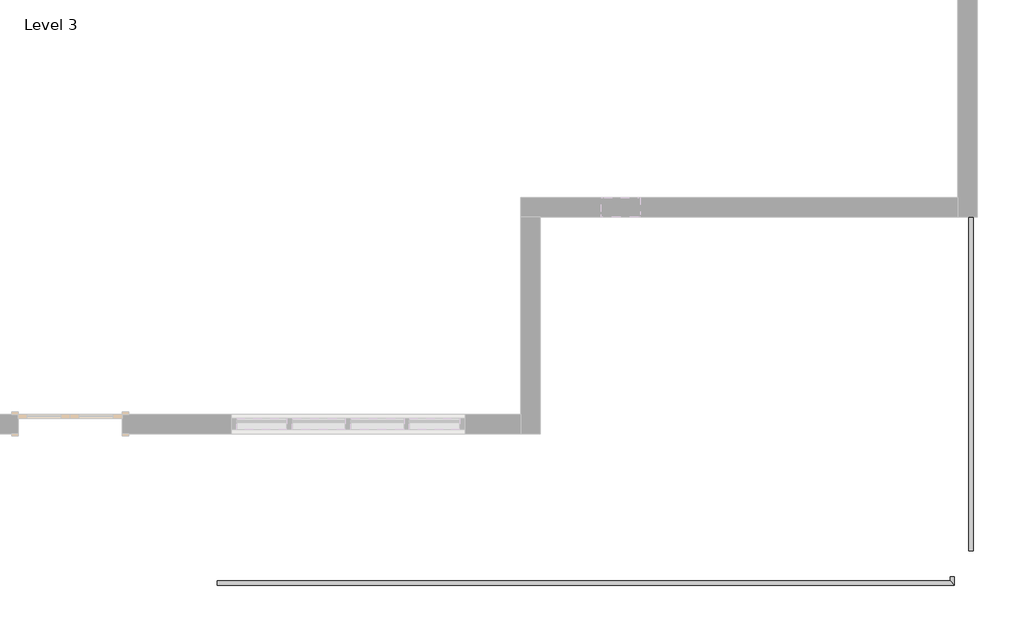
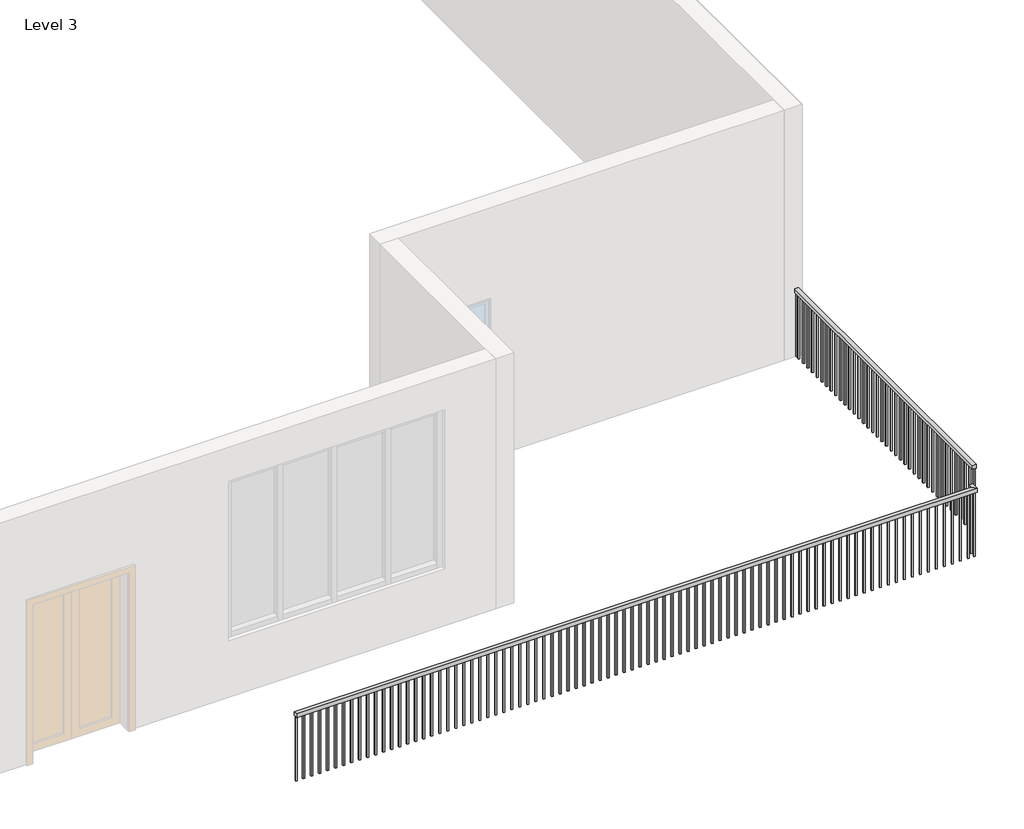
# One storey, part 2 of 2: 2 railings.
"""IFC4 building model written with IfcOpenShell, lengths in millimetres."""

from ifc_helpers import new_model, si_unit, frame, origin, place, context, project, spatial, polyline, outline, extrude, faceted_brep, element, save

model = new_model("IFC4")

# Units and contexts
model_context = context("Model", 3, world=origin())
ifc_project = project(units=[si_unit("LENGTHUNIT", "METRE", prefix="MILLI")], contexts=[model_context])

# Site, building, storey
site = spatial("IfcSite", under=ifc_project)
building = spatial("IfcBuilding", under=site)
storey = spatial("IfcBuildingStorey", under=building, Name="Level 3", Elevation=4114.8)

# Railings
placement = place(None, origin())
element("IfcRailing", 1, ObjectType="Handrail - Rectangular", at=placement, inside=storey, context=model_context, shape_type="SolidModel", body=[
    faceted_brep([(-103.6484006, -4656.0372669, 5029.2), (-103.6484006, -4656.0372669, 4978.4), (-103.6484006, -4706.8372669, 4978.4), (-103.6484006, -4706.8372669, 5029.2), (8481.5515994, -4656.0372669, 5029.2), (8481.5515994, -4656.0372669, 4978.4), (8532.3515994, -4706.8372669, 4978.4), (8532.3515994, -4706.8372669, 5029.2), (8481.5515994, -4605.2372669, 5029.2), (8532.3515994, -4605.2372669, 5029.2), (8532.3515994, -4605.2372669, 4978.4), (8481.5515994, -4605.2372669, 4978.4)], [[[0, 1, 2, 3]], [[1, 0, 4, 5]], [[2, 1, 5, 6]], [[3, 2, 6, 7]], [[0, 3, 7, 4]], [[8, 9, 10, 11]], [[5, 4, 8, 11]], [[6, 5, 11, 10]], [[7, 6, 10, 9]], [[4, 7, 9, 8]]]),
    extrude(outline(polyline([(8421.2265994, -4690.9622669), (8421.2265994, -4671.9122669), (8440.2765994, -4671.9122669), (8440.2765994, -4690.9622669), (8421.2265994, -4690.9622669)])), frame((0.0, 0.0, 4114.8), z_axis=(0.0, 0.0, 1.0), x_axis=(1.0, 0.0, 0.0)), (0.0, 0.0, 1.0), 863.6),
    extrude(outline(polyline([(8319.6265994, -4690.9622669), (8319.6265994, -4671.9122669), (8338.6765994, -4671.9122669), (8338.6765994, -4690.9622669), (8319.6265994, -4690.9622669)])), frame((0.0, 0.0, 4114.8), z_axis=(0.0, 0.0, 1.0), x_axis=(1.0, 0.0, 0.0)), (0.0, 0.0, 1.0), 863.6),
    extrude(outline(polyline([(8218.0265994, -4690.9622669), (8218.0265994, -4671.9122669), (8237.0765994, -4671.9122669), (8237.0765994, -4690.9622669), (8218.0265994, -4690.9622669)])), frame((0.0, 0.0, 4114.8), z_axis=(0.0, 0.0, 1.0), x_axis=(1.0, 0.0, 0.0)), (0.0, 0.0, 1.0), 863.6),
    extrude(outline(polyline([(8116.4265994, -4690.9622669), (8116.4265994, -4671.9122669), (8135.4765994, -4671.9122669), (8135.4765994, -4690.9622669), (8116.4265994, -4690.9622669)])), frame((0.0, 0.0, 4114.8), z_axis=(0.0, 0.0, 1.0), x_axis=(1.0, 0.0, 0.0)), (0.0, 0.0, 1.0), 863.6),
    extrude(outline(polyline([(8014.8265994, -4690.9622669), (8014.8265994, -4671.9122669), (8033.8765994, -4671.9122669), (8033.8765994, -4690.9622669), (8014.8265994, -4690.9622669)])), frame((0.0, 0.0, 4114.8), z_axis=(0.0, 0.0, 1.0), x_axis=(1.0, 0.0, 0.0)), (0.0, 0.0, 1.0), 863.6),
    extrude(outline(polyline([(7913.2265994, -4690.9622669), (7913.2265994, -4671.9122669), (7932.2765994, -4671.9122669), (7932.2765994, -4690.9622669), (7913.2265994, -4690.9622669)])), frame((0.0, 0.0, 4114.8), z_axis=(0.0, 0.0, 1.0), x_axis=(1.0, 0.0, 0.0)), (0.0, 0.0, 1.0), 863.6),
    extrude(outline(polyline([(7811.6265994, -4690.9622669), (7811.6265994, -4671.9122669), (7830.6765994, -4671.9122669), (7830.6765994, -4690.9622669), (7811.6265994, -4690.9622669)])), frame((0.0, 0.0, 4114.8), z_axis=(0.0, 0.0, 1.0), x_axis=(1.0, 0.0, 0.0)), (0.0, 0.0, 1.0), 863.6),
    extrude(outline(polyline([(7710.0265994, -4690.9622669), (7710.0265994, -4671.9122669), (7729.0765994, -4671.9122669), (7729.0765994, -4690.9622669), (7710.0265994, -4690.9622669)])), frame((0.0, 0.0, 4114.8), z_axis=(0.0, 0.0, 1.0), x_axis=(1.0, 0.0, 0.0)), (0.0, 0.0, 1.0), 863.6),
    extrude(outline(polyline([(7608.4265994, -4690.9622669), (7608.4265994, -4671.9122669), (7627.4765994, -4671.9122669), (7627.4765994, -4690.9622669), (7608.4265994, -4690.9622669)])), frame((0.0, 0.0, 4114.8), z_axis=(0.0, 0.0, 1.0), x_axis=(1.0, 0.0, 0.0)), (0.0, 0.0, 1.0), 863.6),
    extrude(outline(polyline([(7506.8265994, -4690.9622669), (7506.8265994, -4671.9122669), (7525.8765994, -4671.9122669), (7525.8765994, -4690.9622669), (7506.8265994, -4690.9622669)])), frame((0.0, 0.0, 4114.8), z_axis=(0.0, 0.0, 1.0), x_axis=(1.0, 0.0, 0.0)), (0.0, 0.0, 1.0), 863.6),
    extrude(outline(polyline([(7405.2265994, -4690.9622669), (7405.2265994, -4671.9122669), (7424.2765994, -4671.9122669), (7424.2765994, -4690.9622669), (7405.2265994, -4690.9622669)])), frame((0.0, 0.0, 4114.8), z_axis=(0.0, 0.0, 1.0), x_axis=(1.0, 0.0, 0.0)), (0.0, 0.0, 1.0), 863.6),
    extrude(outline(polyline([(7303.6265994, -4690.9622669), (7303.6265994, -4671.9122669), (7322.6765994, -4671.9122669), (7322.6765994, -4690.9622669), (7303.6265994, -4690.9622669)])), frame((0.0, 0.0, 4114.8), z_axis=(0.0, 0.0, 1.0), x_axis=(1.0, 0.0, 0.0)), (0.0, 0.0, 1.0), 863.6),
    extrude(outline(polyline([(7202.0265994, -4690.9622669), (7202.0265994, -4671.9122669), (7221.0765994, -4671.9122669), (7221.0765994, -4690.9622669), (7202.0265994, -4690.9622669)])), frame((0.0, 0.0, 4114.8), z_axis=(0.0, 0.0, 1.0), x_axis=(1.0, 0.0, 0.0)), (0.0, 0.0, 1.0), 863.6),
    extrude(outline(polyline([(7100.4265994, -4690.9622669), (7100.4265994, -4671.9122669), (7119.4765994, -4671.9122669), (7119.4765994, -4690.9622669), (7100.4265994, -4690.9622669)])), frame((0.0, 0.0, 4114.8), z_axis=(0.0, 0.0, 1.0), x_axis=(1.0, 0.0, 0.0)), (0.0, 0.0, 1.0), 863.6),
    extrude(outline(polyline([(6998.8265994, -4690.9622669), (6998.8265994, -4671.9122669), (7017.8765994, -4671.9122669), (7017.8765994, -4690.9622669), (6998.8265994, -4690.9622669)])), frame((0.0, 0.0, 4114.8), z_axis=(0.0, 0.0, 1.0), x_axis=(1.0, 0.0, 0.0)), (0.0, 0.0, 1.0), 863.6),
    extrude(outline(polyline([(6897.2265994, -4690.9622669), (6897.2265994, -4671.9122669), (6916.2765994, -4671.9122669), (6916.2765994, -4690.9622669), (6897.2265994, -4690.9622669)])), frame((0.0, 0.0, 4114.8), z_axis=(0.0, 0.0, 1.0), x_axis=(1.0, 0.0, 0.0)), (0.0, 0.0, 1.0), 863.6),
    extrude(outline(polyline([(6795.6265994, -4690.9622669), (6795.6265994, -4671.9122669), (6814.6765994, -4671.9122669), (6814.6765994, -4690.9622669), (6795.6265994, -4690.9622669)])), frame((0.0, 0.0, 4114.8), z_axis=(0.0, 0.0, 1.0), x_axis=(1.0, 0.0, 0.0)), (0.0, 0.0, 1.0), 863.6),
    extrude(outline(polyline([(6694.0265994, -4690.9622669), (6694.0265994, -4671.9122669), (6713.0765994, -4671.9122669), (6713.0765994, -4690.9622669), (6694.0265994, -4690.9622669)])), frame((0.0, 0.0, 4114.8), z_axis=(0.0, 0.0, 1.0), x_axis=(1.0, 0.0, 0.0)), (0.0, 0.0, 1.0), 863.6),
    extrude(outline(polyline([(6592.4265994, -4690.9622669), (6592.4265994, -4671.9122669), (6611.4765994, -4671.9122669), (6611.4765994, -4690.9622669), (6592.4265994, -4690.9622669)])), frame((0.0, 0.0, 4114.8), z_axis=(0.0, 0.0, 1.0), x_axis=(1.0, 0.0, 0.0)), (0.0, 0.0, 1.0), 863.6),
    extrude(outline(polyline([(6490.8265994, -4690.9622669), (6490.8265994, -4671.9122669), (6509.8765994, -4671.9122669), (6509.8765994, -4690.9622669), (6490.8265994, -4690.9622669)])), frame((0.0, 0.0, 4114.8), z_axis=(0.0, 0.0, 1.0), x_axis=(1.0, 0.0, 0.0)), (0.0, 0.0, 1.0), 863.6),
    extrude(outline(polyline([(6389.2265994, -4690.9622669), (6389.2265994, -4671.9122669), (6408.2765994, -4671.9122669), (6408.2765994, -4690.9622669), (6389.2265994, -4690.9622669)])), frame((0.0, 0.0, 4114.8), z_axis=(0.0, 0.0, 1.0), x_axis=(1.0, 0.0, 0.0)), (0.0, 0.0, 1.0), 863.6),
    extrude(outline(polyline([(6287.6265994, -4690.9622669), (6287.6265994, -4671.9122669), (6306.6765994, -4671.9122669), (6306.6765994, -4690.9622669), (6287.6265994, -4690.9622669)])), frame((0.0, 0.0, 4114.8), z_axis=(0.0, 0.0, 1.0), x_axis=(1.0, 0.0, 0.0)), (0.0, 0.0, 1.0), 863.6),
    extrude(outline(polyline([(6186.0265994, -4690.9622669), (6186.0265994, -4671.9122669), (6205.0765994, -4671.9122669), (6205.0765994, -4690.9622669), (6186.0265994, -4690.9622669)])), frame((0.0, 0.0, 4114.8), z_axis=(0.0, 0.0, 1.0), x_axis=(1.0, 0.0, 0.0)), (0.0, 0.0, 1.0), 863.6),
    extrude(outline(polyline([(6084.4265994, -4690.9622669), (6084.4265994, -4671.9122669), (6103.4765994, -4671.9122669), (6103.4765994, -4690.9622669), (6084.4265994, -4690.9622669)])), frame((0.0, 0.0, 4114.8), z_axis=(0.0, 0.0, 1.0), x_axis=(1.0, 0.0, 0.0)), (0.0, 0.0, 1.0), 863.6),
    extrude(outline(polyline([(5982.8265994, -4690.9622669), (5982.8265994, -4671.9122669), (6001.8765994, -4671.9122669), (6001.8765994, -4690.9622669), (5982.8265994, -4690.9622669)])), frame((0.0, 0.0, 4114.8), z_axis=(0.0, 0.0, 1.0), x_axis=(1.0, 0.0, 0.0)), (0.0, 0.0, 1.0), 863.6),
    extrude(outline(polyline([(5881.2265994, -4690.9622669), (5881.2265994, -4671.9122669), (5900.2765994, -4671.9122669), (5900.2765994, -4690.9622669), (5881.2265994, -4690.9622669)])), frame((0.0, 0.0, 4114.8), z_axis=(0.0, 0.0, 1.0), x_axis=(1.0, 0.0, 0.0)), (0.0, 0.0, 1.0), 863.6),
    extrude(outline(polyline([(5779.6265994, -4690.9622669), (5779.6265994, -4671.9122669), (5798.6765994, -4671.9122669), (5798.6765994, -4690.9622669), (5779.6265994, -4690.9622669)])), frame((0.0, 0.0, 4114.8), z_axis=(0.0, 0.0, 1.0), x_axis=(1.0, 0.0, 0.0)), (0.0, 0.0, 1.0), 863.6),
    extrude(outline(polyline([(5678.0265994, -4690.9622669), (5678.0265994, -4671.9122669), (5697.0765994, -4671.9122669), (5697.0765994, -4690.9622669), (5678.0265994, -4690.9622669)])), frame((0.0, 0.0, 4114.8), z_axis=(0.0, 0.0, 1.0), x_axis=(1.0, 0.0, 0.0)), (0.0, 0.0, 1.0), 863.6),
    extrude(outline(polyline([(5576.4265994, -4690.9622669), (5576.4265994, -4671.9122669), (5595.4765994, -4671.9122669), (5595.4765994, -4690.9622669), (5576.4265994, -4690.9622669)])), frame((0.0, 0.0, 4114.8), z_axis=(0.0, 0.0, 1.0), x_axis=(1.0, 0.0, 0.0)), (0.0, 0.0, 1.0), 863.6),
    extrude(outline(polyline([(5474.8265994, -4690.9622669), (5474.8265994, -4671.9122669), (5493.8765994, -4671.9122669), (5493.8765994, -4690.9622669), (5474.8265994, -4690.9622669)])), frame((0.0, 0.0, 4114.8), z_axis=(0.0, 0.0, 1.0), x_axis=(1.0, 0.0, 0.0)), (0.0, 0.0, 1.0), 863.6),
    extrude(outline(polyline([(5373.2265994, -4690.9622669), (5373.2265994, -4671.9122669), (5392.2765994, -4671.9122669), (5392.2765994, -4690.9622669), (5373.2265994, -4690.9622669)])), frame((0.0, 0.0, 4114.8), z_axis=(0.0, 0.0, 1.0), x_axis=(1.0, 0.0, 0.0)), (0.0, 0.0, 1.0), 863.6),
    extrude(outline(polyline([(5271.6265994, -4690.9622669), (5271.6265994, -4671.9122669), (5290.6765994, -4671.9122669), (5290.6765994, -4690.9622669), (5271.6265994, -4690.9622669)])), frame((0.0, 0.0, 4114.8), z_axis=(0.0, 0.0, 1.0), x_axis=(1.0, 0.0, 0.0)), (0.0, 0.0, 1.0), 863.6),
    extrude(outline(polyline([(5170.0265994, -4690.9622669), (5170.0265994, -4671.9122669), (5189.0765994, -4671.9122669), (5189.0765994, -4690.9622669), (5170.0265994, -4690.9622669)])), frame((0.0, 0.0, 4114.8), z_axis=(0.0, 0.0, 1.0), x_axis=(1.0, 0.0, 0.0)), (0.0, 0.0, 1.0), 863.6),
    extrude(outline(polyline([(5068.4265994, -4690.9622669), (5068.4265994, -4671.9122669), (5087.4765994, -4671.9122669), (5087.4765994, -4690.9622669), (5068.4265994, -4690.9622669)])), frame((0.0, 0.0, 4114.8), z_axis=(0.0, 0.0, 1.0), x_axis=(1.0, 0.0, 0.0)), (0.0, 0.0, 1.0), 863.6),
    extrude(outline(polyline([(4966.8265994, -4690.9622669), (4966.8265994, -4671.9122669), (4985.8765994, -4671.9122669), (4985.8765994, -4690.9622669), (4966.8265994, -4690.9622669)])), frame((0.0, 0.0, 4114.8), z_axis=(0.0, 0.0, 1.0), x_axis=(1.0, 0.0, 0.0)), (0.0, 0.0, 1.0), 863.6),
    extrude(outline(polyline([(4865.2265994, -4690.9622669), (4865.2265994, -4671.9122669), (4884.2765994, -4671.9122669), (4884.2765994, -4690.9622669), (4865.2265994, -4690.9622669)])), frame((0.0, 0.0, 4114.8), z_axis=(0.0, 0.0, 1.0), x_axis=(1.0, 0.0, 0.0)), (0.0, 0.0, 1.0), 863.6),
    extrude(outline(polyline([(4763.6265994, -4690.9622669), (4763.6265994, -4671.9122669), (4782.6765994, -4671.9122669), (4782.6765994, -4690.9622669), (4763.6265994, -4690.9622669)])), frame((0.0, 0.0, 4114.8), z_axis=(0.0, 0.0, 1.0), x_axis=(1.0, 0.0, 0.0)), (0.0, 0.0, 1.0), 863.6),
    extrude(outline(polyline([(4662.0265994, -4690.9622669), (4662.0265994, -4671.9122669), (4681.0765994, -4671.9122669), (4681.0765994, -4690.9622669), (4662.0265994, -4690.9622669)])), frame((0.0, 0.0, 4114.8), z_axis=(0.0, 0.0, 1.0), x_axis=(1.0, 0.0, 0.0)), (0.0, 0.0, 1.0), 863.6),
    extrude(outline(polyline([(4560.4265994, -4690.9622669), (4560.4265994, -4671.9122669), (4579.4765994, -4671.9122669), (4579.4765994, -4690.9622669), (4560.4265994, -4690.9622669)])), frame((0.0, 0.0, 4114.8), z_axis=(0.0, 0.0, 1.0), x_axis=(1.0, 0.0, 0.0)), (0.0, 0.0, 1.0), 863.6),
    extrude(outline(polyline([(4458.8265994, -4690.9622669), (4458.8265994, -4671.9122669), (4477.8765994, -4671.9122669), (4477.8765994, -4690.9622669), (4458.8265994, -4690.9622669)])), frame((0.0, 0.0, 4114.8), z_axis=(0.0, 0.0, 1.0), x_axis=(1.0, 0.0, 0.0)), (0.0, 0.0, 1.0), 863.6),
    extrude(outline(polyline([(4357.2265994, -4690.9622669), (4357.2265994, -4671.9122669), (4376.2765994, -4671.9122669), (4376.2765994, -4690.9622669), (4357.2265994, -4690.9622669)])), frame((0.0, 0.0, 4114.8), z_axis=(0.0, 0.0, 1.0), x_axis=(1.0, 0.0, 0.0)), (0.0, 0.0, 1.0), 863.6),
    extrude(outline(polyline([(4255.6265994, -4690.9622669), (4255.6265994, -4671.9122669), (4274.6765994, -4671.9122669), (4274.6765994, -4690.9622669), (4255.6265994, -4690.9622669)])), frame((0.0, 0.0, 4114.8), z_axis=(0.0, 0.0, 1.0), x_axis=(1.0, 0.0, 0.0)), (0.0, 0.0, 1.0), 863.6),
    extrude(outline(polyline([(4154.0265994, -4690.9622669), (4154.0265994, -4671.9122669), (4173.0765994, -4671.9122669), (4173.0765994, -4690.9622669), (4154.0265994, -4690.9622669)])), frame((0.0, 0.0, 4114.8), z_axis=(0.0, 0.0, 1.0), x_axis=(1.0, 0.0, 0.0)), (0.0, 0.0, 1.0), 863.6),
    extrude(outline(polyline([(4052.4265994, -4690.9622669), (4052.4265994, -4671.9122669), (4071.4765994, -4671.9122669), (4071.4765994, -4690.9622669), (4052.4265994, -4690.9622669)])), frame((0.0, 0.0, 4114.8), z_axis=(0.0, 0.0, 1.0), x_axis=(1.0, 0.0, 0.0)), (0.0, 0.0, 1.0), 863.6),
    extrude(outline(polyline([(3950.8265994, -4690.9622669), (3950.8265994, -4671.9122669), (3969.8765994, -4671.9122669), (3969.8765994, -4690.9622669), (3950.8265994, -4690.9622669)])), frame((0.0, 0.0, 4114.8), z_axis=(0.0, 0.0, 1.0), x_axis=(1.0, 0.0, 0.0)), (0.0, 0.0, 1.0), 863.6),
    extrude(outline(polyline([(3849.2265994, -4690.9622669), (3849.2265994, -4671.9122669), (3868.2765994, -4671.9122669), (3868.2765994, -4690.9622669), (3849.2265994, -4690.9622669)])), frame((0.0, 0.0, 4114.8), z_axis=(0.0, 0.0, 1.0), x_axis=(1.0, 0.0, 0.0)), (0.0, 0.0, 1.0), 863.6),
    extrude(outline(polyline([(3747.6265994, -4690.9622669), (3747.6265994, -4671.9122669), (3766.6765994, -4671.9122669), (3766.6765994, -4690.9622669), (3747.6265994, -4690.9622669)])), frame((0.0, 0.0, 4114.8), z_axis=(0.0, 0.0, 1.0), x_axis=(1.0, 0.0, 0.0)), (0.0, 0.0, 1.0), 863.6),
    extrude(outline(polyline([(3646.0265994, -4690.9622669), (3646.0265994, -4671.9122669), (3665.0765994, -4671.9122669), (3665.0765994, -4690.9622669), (3646.0265994, -4690.9622669)])), frame((0.0, 0.0, 4114.8), z_axis=(0.0, 0.0, 1.0), x_axis=(1.0, 0.0, 0.0)), (0.0, 0.0, 1.0), 863.6),
    extrude(outline(polyline([(3544.4265994, -4690.9622669), (3544.4265994, -4671.9122669), (3563.4765994, -4671.9122669), (3563.4765994, -4690.9622669), (3544.4265994, -4690.9622669)])), frame((0.0, 0.0, 4114.8), z_axis=(0.0, 0.0, 1.0), x_axis=(1.0, 0.0, 0.0)), (0.0, 0.0, 1.0), 863.6),
    extrude(outline(polyline([(3442.8265994, -4690.9622669), (3442.8265994, -4671.9122669), (3461.8765994, -4671.9122669), (3461.8765994, -4690.9622669), (3442.8265994, -4690.9622669)])), frame((0.0, 0.0, 4114.8), z_axis=(0.0, 0.0, 1.0), x_axis=(1.0, 0.0, 0.0)), (0.0, 0.0, 1.0), 863.6),
    extrude(outline(polyline([(3341.2265994, -4690.9622669), (3341.2265994, -4671.9122669), (3360.2765994, -4671.9122669), (3360.2765994, -4690.9622669), (3341.2265994, -4690.9622669)])), frame((0.0, 0.0, 4114.8), z_axis=(0.0, 0.0, 1.0), x_axis=(1.0, 0.0, 0.0)), (0.0, 0.0, 1.0), 863.6),
    extrude(outline(polyline([(3239.6265994, -4690.9622669), (3239.6265994, -4671.9122669), (3258.6765994, -4671.9122669), (3258.6765994, -4690.9622669), (3239.6265994, -4690.9622669)])), frame((0.0, 0.0, 4114.8), z_axis=(0.0, 0.0, 1.0), x_axis=(1.0, 0.0, 0.0)), (0.0, 0.0, 1.0), 863.6),
    extrude(outline(polyline([(3138.0265994, -4690.9622669), (3138.0265994, -4671.9122669), (3157.0765994, -4671.9122669), (3157.0765994, -4690.9622669), (3138.0265994, -4690.9622669)])), frame((0.0, 0.0, 4114.8), z_axis=(0.0, 0.0, 1.0), x_axis=(1.0, 0.0, 0.0)), (0.0, 0.0, 1.0), 863.6),
    extrude(outline(polyline([(3036.4265994, -4690.9622669), (3036.4265994, -4671.9122669), (3055.4765994, -4671.9122669), (3055.4765994, -4690.9622669), (3036.4265994, -4690.9622669)])), frame((0.0, 0.0, 4114.8), z_axis=(0.0, 0.0, 1.0), x_axis=(1.0, 0.0, 0.0)), (0.0, 0.0, 1.0), 863.6),
    extrude(outline(polyline([(2934.8265994, -4690.9622669), (2934.8265994, -4671.9122669), (2953.8765994, -4671.9122669), (2953.8765994, -4690.9622669), (2934.8265994, -4690.9622669)])), frame((0.0, 0.0, 4114.8), z_axis=(0.0, 0.0, 1.0), x_axis=(1.0, 0.0, 0.0)), (0.0, 0.0, 1.0), 863.6),
    extrude(outline(polyline([(2833.2265994, -4690.9622669), (2833.2265994, -4671.9122669), (2852.2765994, -4671.9122669), (2852.2765994, -4690.9622669), (2833.2265994, -4690.9622669)])), frame((0.0, 0.0, 4114.8), z_axis=(0.0, 0.0, 1.0), x_axis=(1.0, 0.0, 0.0)), (0.0, 0.0, 1.0), 863.6),
    extrude(outline(polyline([(2731.6265994, -4690.9622669), (2731.6265994, -4671.9122669), (2750.6765994, -4671.9122669), (2750.6765994, -4690.9622669), (2731.6265994, -4690.9622669)])), frame((0.0, 0.0, 4114.8), z_axis=(0.0, 0.0, 1.0), x_axis=(1.0, 0.0, 0.0)), (0.0, 0.0, 1.0), 863.6),
    extrude(outline(polyline([(2630.0265994, -4690.9622669), (2630.0265994, -4671.9122669), (2649.0765994, -4671.9122669), (2649.0765994, -4690.9622669), (2630.0265994, -4690.9622669)])), frame((0.0, 0.0, 4114.8), z_axis=(0.0, 0.0, 1.0), x_axis=(1.0, 0.0, 0.0)), (0.0, 0.0, 1.0), 863.6),
    extrude(outline(polyline([(2528.4265994, -4690.9622669), (2528.4265994, -4671.9122669), (2547.4765994, -4671.9122669), (2547.4765994, -4690.9622669), (2528.4265994, -4690.9622669)])), frame((0.0, 0.0, 4114.8), z_axis=(0.0, 0.0, 1.0), x_axis=(1.0, 0.0, 0.0)), (0.0, 0.0, 1.0), 863.6),
    extrude(outline(polyline([(2426.8265994, -4690.9622669), (2426.8265994, -4671.9122669), (2445.8765994, -4671.9122669), (2445.8765994, -4690.9622669), (2426.8265994, -4690.9622669)])), frame((0.0, 0.0, 4114.8), z_axis=(0.0, 0.0, 1.0), x_axis=(1.0, 0.0, 0.0)), (0.0, 0.0, 1.0), 863.6),
    extrude(outline(polyline([(2325.2265994, -4690.9622669), (2325.2265994, -4671.9122669), (2344.2765994, -4671.9122669), (2344.2765994, -4690.9622669), (2325.2265994, -4690.9622669)])), frame((0.0, 0.0, 4114.8), z_axis=(0.0, 0.0, 1.0), x_axis=(1.0, 0.0, 0.0)), (0.0, 0.0, 1.0), 863.6),
    extrude(outline(polyline([(2223.6265994, -4690.9622669), (2223.6265994, -4671.9122669), (2242.6765994, -4671.9122669), (2242.6765994, -4690.9622669), (2223.6265994, -4690.9622669)])), frame((0.0, 0.0, 4114.8), z_axis=(0.0, 0.0, 1.0), x_axis=(1.0, 0.0, 0.0)), (0.0, 0.0, 1.0), 863.6),
    extrude(outline(polyline([(2122.0265994, -4690.9622669), (2122.0265994, -4671.9122669), (2141.0765994, -4671.9122669), (2141.0765994, -4690.9622669), (2122.0265994, -4690.9622669)])), frame((0.0, 0.0, 4114.8), z_axis=(0.0, 0.0, 1.0), x_axis=(1.0, 0.0, 0.0)), (0.0, 0.0, 1.0), 863.6),
    extrude(outline(polyline([(2020.4265994, -4690.9622669), (2020.4265994, -4671.9122669), (2039.4765994, -4671.9122669), (2039.4765994, -4690.9622669), (2020.4265994, -4690.9622669)])), frame((0.0, 0.0, 4114.8), z_axis=(0.0, 0.0, 1.0), x_axis=(1.0, 0.0, 0.0)), (0.0, 0.0, 1.0), 863.6),
    extrude(outline(polyline([(1918.8265994, -4690.9622669), (1918.8265994, -4671.9122669), (1937.8765994, -4671.9122669), (1937.8765994, -4690.9622669), (1918.8265994, -4690.9622669)])), frame((0.0, 0.0, 4114.8), z_axis=(0.0, 0.0, 1.0), x_axis=(1.0, 0.0, 0.0)), (0.0, 0.0, 1.0), 863.6),
    extrude(outline(polyline([(1817.2265994, -4690.9622669), (1817.2265994, -4671.9122669), (1836.2765994, -4671.9122669), (1836.2765994, -4690.9622669), (1817.2265994, -4690.9622669)])), frame((0.0, 0.0, 4114.8), z_axis=(0.0, 0.0, 1.0), x_axis=(1.0, 0.0, 0.0)), (0.0, 0.0, 1.0), 863.6),
    extrude(outline(polyline([(1715.6265994, -4690.9622669), (1715.6265994, -4671.9122669), (1734.6765994, -4671.9122669), (1734.6765994, -4690.9622669), (1715.6265994, -4690.9622669)])), frame((0.0, 0.0, 4114.8), z_axis=(0.0, 0.0, 1.0), x_axis=(1.0, 0.0, 0.0)), (0.0, 0.0, 1.0), 863.6),
    extrude(outline(polyline([(1614.0265994, -4690.9622669), (1614.0265994, -4671.9122669), (1633.0765994, -4671.9122669), (1633.0765994, -4690.9622669), (1614.0265994, -4690.9622669)])), frame((0.0, 0.0, 4114.8), z_axis=(0.0, 0.0, 1.0), x_axis=(1.0, 0.0, 0.0)), (0.0, 0.0, 1.0), 863.6),
    extrude(outline(polyline([(1512.4265994, -4690.9622669), (1512.4265994, -4671.9122669), (1531.4765994, -4671.9122669), (1531.4765994, -4690.9622669), (1512.4265994, -4690.9622669)])), frame((0.0, 0.0, 4114.8), z_axis=(0.0, 0.0, 1.0), x_axis=(1.0, 0.0, 0.0)), (0.0, 0.0, 1.0), 863.6),
    extrude(outline(polyline([(1410.8265994, -4690.9622669), (1410.8265994, -4671.9122669), (1429.8765994, -4671.9122669), (1429.8765994, -4690.9622669), (1410.8265994, -4690.9622669)])), frame((0.0, 0.0, 4114.8), z_axis=(0.0, 0.0, 1.0), x_axis=(1.0, 0.0, 0.0)), (0.0, 0.0, 1.0), 863.6),
    extrude(outline(polyline([(1309.2265994, -4690.9622669), (1309.2265994, -4671.9122669), (1328.2765994, -4671.9122669), (1328.2765994, -4690.9622669), (1309.2265994, -4690.9622669)])), frame((0.0, 0.0, 4114.8), z_axis=(0.0, 0.0, 1.0), x_axis=(1.0, 0.0, 0.0)), (0.0, 0.0, 1.0), 863.6),
    extrude(outline(polyline([(1207.6265994, -4690.9622669), (1207.6265994, -4671.9122669), (1226.6765994, -4671.9122669), (1226.6765994, -4690.9622669), (1207.6265994, -4690.9622669)])), frame((0.0, 0.0, 4114.8), z_axis=(0.0, 0.0, 1.0), x_axis=(1.0, 0.0, 0.0)), (0.0, 0.0, 1.0), 863.6),
    extrude(outline(polyline([(1106.0265994, -4690.9622669), (1106.0265994, -4671.9122669), (1125.0765994, -4671.9122669), (1125.0765994, -4690.9622669), (1106.0265994, -4690.9622669)])), frame((0.0, 0.0, 4114.8), z_axis=(0.0, 0.0, 1.0), x_axis=(1.0, 0.0, 0.0)), (0.0, 0.0, 1.0), 863.6),
    extrude(outline(polyline([(1004.4265994, -4690.9622669), (1004.4265994, -4671.9122669), (1023.4765994, -4671.9122669), (1023.4765994, -4690.9622669), (1004.4265994, -4690.9622669)])), frame((0.0, 0.0, 4114.8), z_axis=(0.0, 0.0, 1.0), x_axis=(1.0, 0.0, 0.0)), (0.0, 0.0, 1.0), 863.6),
    extrude(outline(polyline([(902.8265994, -4690.9622669), (902.8265994, -4671.9122669), (921.8765994, -4671.9122669), (921.8765994, -4690.9622669), (902.8265994, -4690.9622669)])), frame((0.0, 0.0, 4114.8), z_axis=(0.0, 0.0, 1.0), x_axis=(1.0, 0.0, 0.0)), (0.0, 0.0, 1.0), 863.6),
    extrude(outline(polyline([(801.2265994, -4690.9622669), (801.2265994, -4671.9122669), (820.2765994, -4671.9122669), (820.2765994, -4690.9622669), (801.2265994, -4690.9622669)])), frame((0.0, 0.0, 4114.8), z_axis=(0.0, 0.0, 1.0), x_axis=(1.0, 0.0, 0.0)), (0.0, 0.0, 1.0), 863.6),
    extrude(outline(polyline([(699.6265994, -4690.9622669), (699.6265994, -4671.9122669), (718.6765994, -4671.9122669), (718.6765994, -4690.9622669), (699.6265994, -4690.9622669)])), frame((0.0, 0.0, 4114.8), z_axis=(0.0, 0.0, 1.0), x_axis=(1.0, 0.0, 0.0)), (0.0, 0.0, 1.0), 863.6),
    extrude(outline(polyline([(598.0265994, -4690.9622669), (598.0265994, -4671.9122669), (617.0765994, -4671.9122669), (617.0765994, -4690.9622669), (598.0265994, -4690.9622669)])), frame((0.0, 0.0, 4114.8), z_axis=(0.0, 0.0, 1.0), x_axis=(1.0, 0.0, 0.0)), (0.0, 0.0, 1.0), 863.6),
    extrude(outline(polyline([(496.4265994, -4690.9622669), (496.4265994, -4671.9122669), (515.4765994, -4671.9122669), (515.4765994, -4690.9622669), (496.4265994, -4690.9622669)])), frame((0.0, 0.0, 4114.8), z_axis=(0.0, 0.0, 1.0), x_axis=(1.0, 0.0, 0.0)), (0.0, 0.0, 1.0), 863.6),
    extrude(outline(polyline([(394.8265994, -4690.9622669), (394.8265994, -4671.9122669), (413.8765994, -4671.9122669), (413.8765994, -4690.9622669), (394.8265994, -4690.9622669)])), frame((0.0, 0.0, 4114.8), z_axis=(0.0, 0.0, 1.0), x_axis=(1.0, 0.0, 0.0)), (0.0, 0.0, 1.0), 863.6),
    extrude(outline(polyline([(293.2265994, -4690.9622669), (293.2265994, -4671.9122669), (312.2765994, -4671.9122669), (312.2765994, -4690.9622669), (293.2265994, -4690.9622669)])), frame((0.0, 0.0, 4114.8), z_axis=(0.0, 0.0, 1.0), x_axis=(1.0, 0.0, 0.0)), (0.0, 0.0, 1.0), 863.6),
    extrude(outline(polyline([(191.6265994, -4690.9622669), (191.6265994, -4671.9122669), (210.6765994, -4671.9122669), (210.6765994, -4690.9622669), (191.6265994, -4690.9622669)])), frame((0.0, 0.0, 4114.8), z_axis=(0.0, 0.0, 1.0), x_axis=(1.0, 0.0, 0.0)), (0.0, 0.0, 1.0), 863.6),
    extrude(outline(polyline([(90.0265994, -4690.9622669), (90.0265994, -4671.9122669), (109.0765994, -4671.9122669), (109.0765994, -4690.9622669), (90.0265994, -4690.9622669)])), frame((0.0, 0.0, 4114.8), z_axis=(0.0, 0.0, 1.0), x_axis=(1.0, 0.0, 0.0)), (0.0, 0.0, 1.0), 863.6),
    extrude(outline(polyline([(-11.5734006, -4690.9622669), (-11.5734006, -4671.9122669), (7.4765994, -4671.9122669), (7.4765994, -4690.9622669), (-11.5734006, -4690.9622669)])), frame((0.0, 0.0, 4114.8), z_axis=(0.0, 0.0, 1.0), x_axis=(1.0, 0.0, 0.0)), (0.0, 0.0, 1.0), 863.6),
    extrude(outline(polyline([(8497.4265994, -4690.9622669), (8497.4265994, -4671.9122669), (8516.4765994, -4671.9122669), (8516.4765994, -4690.9622669), (8497.4265994, -4690.9622669)])), frame((0.0, 0.0, 4114.8), z_axis=(0.0, 0.0, 1.0), x_axis=(1.0, 0.0, 0.0)), (0.0, 0.0, 1.0), 863.6),
    extrude(outline(polyline([(8516.4765994, -4624.2872669), (8497.4265994, -4624.2872669), (8497.4265994, -4605.2372669), (8516.4765994, -4605.2372669), (8516.4765994, -4624.2872669)])), frame((0.0, 0.0, 4114.8), z_axis=(0.0, 0.0, 1.0), x_axis=(1.0, 0.0, 0.0)), (0.0, 0.0, 1.0), 863.6),
    extrude(outline(polyline([(-103.6484006, -4690.9622669), (-103.6484006, -4671.9122669), (-84.5984006, -4671.9122669), (-84.5984006, -4690.9622669), (-103.6484006, -4690.9622669)])), frame((0.0, 0.0, 4114.8), z_axis=(0.0, 0.0, 1.0), x_axis=(1.0, 0.0, 0.0)), (0.0, 0.0, 1.0), 863.6),
])
element("IfcRailing", 2, ObjectType="Handrail - Rectangular", at=placement, inside=storey, context=model_context, shape_type="SweptSolid", body=[
    extrude(outline(polyline([(8753.8598849, -4300.4372669), (8703.0598849, -4300.4372669), (8703.0598849, -388.8372669), (8753.8598849, -388.8372669), (8753.8598849, -4300.4372669)])), frame((0.0, 0.0, 4978.4), z_axis=(0.0, 0.0, 1.0), x_axis=(1.0, 0.0, 0.0)), (0.0, 0.0, 1.0), 50.8),
    extrude(outline(polyline([(8737.9848849, -449.1622669), (8718.9348849, -449.1622669), (8718.9348849, -430.1122669), (8737.9848849, -430.1122669), (8737.9848849, -449.1622669)])), frame((0.0, 0.0, 4114.8), z_axis=(0.0, 0.0, 1.0), x_axis=(1.0, 0.0, 0.0)), (0.0, 0.0, 1.0), 863.6),
    extrude(outline(polyline([(8737.9848849, -550.7622669), (8718.9348849, -550.7622669), (8718.9348849, -531.7122669), (8737.9848849, -531.7122669), (8737.9848849, -550.7622669)])), frame((0.0, 0.0, 4114.8), z_axis=(0.0, 0.0, 1.0), x_axis=(1.0, 0.0, 0.0)), (0.0, 0.0, 1.0), 863.6),
    extrude(outline(polyline([(8737.9848849, -652.3622669), (8718.9348849, -652.3622669), (8718.9348849, -633.3122669), (8737.9848849, -633.3122669), (8737.9848849, -652.3622669)])), frame((0.0, 0.0, 4114.8), z_axis=(0.0, 0.0, 1.0), x_axis=(1.0, 0.0, 0.0)), (0.0, 0.0, 1.0), 863.6),
    extrude(outline(polyline([(8737.9848849, -753.9622669), (8718.9348849, -753.9622669), (8718.9348849, -734.9122669), (8737.9848849, -734.9122669), (8737.9848849, -753.9622669)])), frame((0.0, 0.0, 4114.8), z_axis=(0.0, 0.0, 1.0), x_axis=(1.0, 0.0, 0.0)), (0.0, 0.0, 1.0), 863.6),
    extrude(outline(polyline([(8737.9848849, -855.5622669), (8718.9348849, -855.5622669), (8718.9348849, -836.5122669), (8737.9848849, -836.5122669), (8737.9848849, -855.5622669)])), frame((0.0, 0.0, 4114.8), z_axis=(0.0, 0.0, 1.0), x_axis=(1.0, 0.0, 0.0)), (0.0, 0.0, 1.0), 863.6),
    extrude(outline(polyline([(8737.9848849, -957.1622669), (8718.9348849, -957.1622669), (8718.9348849, -938.1122669), (8737.9848849, -938.1122669), (8737.9848849, -957.1622669)])), frame((0.0, 0.0, 4114.8), z_axis=(0.0, 0.0, 1.0), x_axis=(1.0, 0.0, 0.0)), (0.0, 0.0, 1.0), 863.6),
    extrude(outline(polyline([(8737.9848849, -1058.7622669), (8718.9348849, -1058.7622669), (8718.9348849, -1039.7122669), (8737.9848849, -1039.7122669), (8737.9848849, -1058.7622669)])), frame((0.0, 0.0, 4114.8), z_axis=(0.0, 0.0, 1.0), x_axis=(1.0, 0.0, 0.0)), (0.0, 0.0, 1.0), 863.6),
    extrude(outline(polyline([(8737.9848849, -1160.3622669), (8718.9348849, -1160.3622669), (8718.9348849, -1141.3122669), (8737.9848849, -1141.3122669), (8737.9848849, -1160.3622669)])), frame((0.0, 0.0, 4114.8), z_axis=(0.0, 0.0, 1.0), x_axis=(1.0, 0.0, 0.0)), (0.0, 0.0, 1.0), 863.6),
    extrude(outline(polyline([(8737.9848849, -1261.9622669), (8718.9348849, -1261.9622669), (8718.9348849, -1242.9122669), (8737.9848849, -1242.9122669), (8737.9848849, -1261.9622669)])), frame((0.0, 0.0, 4114.8), z_axis=(0.0, 0.0, 1.0), x_axis=(1.0, 0.0, 0.0)), (0.0, 0.0, 1.0), 863.6),
    extrude(outline(polyline([(8737.9848849, -1363.5622669), (8718.9348849, -1363.5622669), (8718.9348849, -1344.5122669), (8737.9848849, -1344.5122669), (8737.9848849, -1363.5622669)])), frame((0.0, 0.0, 4114.8), z_axis=(0.0, 0.0, 1.0), x_axis=(1.0, 0.0, 0.0)), (0.0, 0.0, 1.0), 863.6),
    extrude(outline(polyline([(8737.9848849, -1465.1622669), (8718.9348849, -1465.1622669), (8718.9348849, -1446.1122669), (8737.9848849, -1446.1122669), (8737.9848849, -1465.1622669)])), frame((0.0, 0.0, 4114.8), z_axis=(0.0, 0.0, 1.0), x_axis=(1.0, 0.0, 0.0)), (0.0, 0.0, 1.0), 863.6),
    extrude(outline(polyline([(8737.9848849, -1566.7622669), (8718.9348849, -1566.7622669), (8718.9348849, -1547.7122669), (8737.9848849, -1547.7122669), (8737.9848849, -1566.7622669)])), frame((0.0, 0.0, 4114.8), z_axis=(0.0, 0.0, 1.0), x_axis=(1.0, 0.0, 0.0)), (0.0, 0.0, 1.0), 863.6),
    extrude(outline(polyline([(8737.9848849, -1668.3622669), (8718.9348849, -1668.3622669), (8718.9348849, -1649.3122669), (8737.9848849, -1649.3122669), (8737.9848849, -1668.3622669)])), frame((0.0, 0.0, 4114.8), z_axis=(0.0, 0.0, 1.0), x_axis=(1.0, 0.0, 0.0)), (0.0, 0.0, 1.0), 863.6),
    extrude(outline(polyline([(8737.9848849, -1769.9622669), (8718.9348849, -1769.9622669), (8718.9348849, -1750.9122669), (8737.9848849, -1750.9122669), (8737.9848849, -1769.9622669)])), frame((0.0, 0.0, 4114.8), z_axis=(0.0, 0.0, 1.0), x_axis=(1.0, 0.0, 0.0)), (0.0, 0.0, 1.0), 863.6),
    extrude(outline(polyline([(8737.9848849, -1871.5622669), (8718.9348849, -1871.5622669), (8718.9348849, -1852.5122669), (8737.9848849, -1852.5122669), (8737.9848849, -1871.5622669)])), frame((0.0, 0.0, 4114.8), z_axis=(0.0, 0.0, 1.0), x_axis=(1.0, 0.0, 0.0)), (0.0, 0.0, 1.0), 863.6),
    extrude(outline(polyline([(8737.9848849, -1973.1622669), (8718.9348849, -1973.1622669), (8718.9348849, -1954.1122669), (8737.9848849, -1954.1122669), (8737.9848849, -1973.1622669)])), frame((0.0, 0.0, 4114.8), z_axis=(0.0, 0.0, 1.0), x_axis=(1.0, 0.0, 0.0)), (0.0, 0.0, 1.0), 863.6),
    extrude(outline(polyline([(8737.9848849, -2074.7622669), (8718.9348849, -2074.7622669), (8718.9348849, -2055.7122669), (8737.9848849, -2055.7122669), (8737.9848849, -2074.7622669)])), frame((0.0, 0.0, 4114.8), z_axis=(0.0, 0.0, 1.0), x_axis=(1.0, 0.0, 0.0)), (0.0, 0.0, 1.0), 863.6),
    extrude(outline(polyline([(8737.9848849, -2176.3622669), (8718.9348849, -2176.3622669), (8718.9348849, -2157.3122669), (8737.9848849, -2157.3122669), (8737.9848849, -2176.3622669)])), frame((0.0, 0.0, 4114.8), z_axis=(0.0, 0.0, 1.0), x_axis=(1.0, 0.0, 0.0)), (0.0, 0.0, 1.0), 863.6),
    extrude(outline(polyline([(8737.9848849, -2277.9622669), (8718.9348849, -2277.9622669), (8718.9348849, -2258.9122669), (8737.9848849, -2258.9122669), (8737.9848849, -2277.9622669)])), frame((0.0, 0.0, 4114.8), z_axis=(0.0, 0.0, 1.0), x_axis=(1.0, 0.0, 0.0)), (0.0, 0.0, 1.0), 863.6),
    extrude(outline(polyline([(8737.9848849, -2379.5622669), (8718.9348849, -2379.5622669), (8718.9348849, -2360.5122669), (8737.9848849, -2360.5122669), (8737.9848849, -2379.5622669)])), frame((0.0, 0.0, 4114.8), z_axis=(0.0, 0.0, 1.0), x_axis=(1.0, 0.0, 0.0)), (0.0, 0.0, 1.0), 863.6),
    extrude(outline(polyline([(8737.9848849, -2481.1622669), (8718.9348849, -2481.1622669), (8718.9348849, -2462.1122669), (8737.9848849, -2462.1122669), (8737.9848849, -2481.1622669)])), frame((0.0, 0.0, 4114.8), z_axis=(0.0, 0.0, 1.0), x_axis=(1.0, 0.0, 0.0)), (0.0, 0.0, 1.0), 863.6),
    extrude(outline(polyline([(8737.9848849, -2582.7622669), (8718.9348849, -2582.7622669), (8718.9348849, -2563.7122669), (8737.9848849, -2563.7122669), (8737.9848849, -2582.7622669)])), frame((0.0, 0.0, 4114.8), z_axis=(0.0, 0.0, 1.0), x_axis=(1.0, 0.0, 0.0)), (0.0, 0.0, 1.0), 863.6),
    extrude(outline(polyline([(8737.9848849, -2684.3622669), (8718.9348849, -2684.3622669), (8718.9348849, -2665.3122669), (8737.9848849, -2665.3122669), (8737.9848849, -2684.3622669)])), frame((0.0, 0.0, 4114.8), z_axis=(0.0, 0.0, 1.0), x_axis=(1.0, 0.0, 0.0)), (0.0, 0.0, 1.0), 863.6),
    extrude(outline(polyline([(8737.9848849, -2785.9622669), (8718.9348849, -2785.9622669), (8718.9348849, -2766.9122669), (8737.9848849, -2766.9122669), (8737.9848849, -2785.9622669)])), frame((0.0, 0.0, 4114.8), z_axis=(0.0, 0.0, 1.0), x_axis=(1.0, 0.0, 0.0)), (0.0, 0.0, 1.0), 863.6),
    extrude(outline(polyline([(8737.9848849, -2887.5622669), (8718.9348849, -2887.5622669), (8718.9348849, -2868.5122669), (8737.9848849, -2868.5122669), (8737.9848849, -2887.5622669)])), frame((0.0, 0.0, 4114.8), z_axis=(0.0, 0.0, 1.0), x_axis=(1.0, 0.0, 0.0)), (0.0, 0.0, 1.0), 863.6),
    extrude(outline(polyline([(8737.9848849, -2989.1622669), (8718.9348849, -2989.1622669), (8718.9348849, -2970.1122669), (8737.9848849, -2970.1122669), (8737.9848849, -2989.1622669)])), frame((0.0, 0.0, 4114.8), z_axis=(0.0, 0.0, 1.0), x_axis=(1.0, 0.0, 0.0)), (0.0, 0.0, 1.0), 863.6),
    extrude(outline(polyline([(8737.9848849, -3090.7622669), (8718.9348849, -3090.7622669), (8718.9348849, -3071.7122669), (8737.9848849, -3071.7122669), (8737.9848849, -3090.7622669)])), frame((0.0, 0.0, 4114.8), z_axis=(0.0, 0.0, 1.0), x_axis=(1.0, 0.0, 0.0)), (0.0, 0.0, 1.0), 863.6),
    extrude(outline(polyline([(8737.9848849, -3192.3622669), (8718.9348849, -3192.3622669), (8718.9348849, -3173.3122669), (8737.9848849, -3173.3122669), (8737.9848849, -3192.3622669)])), frame((0.0, 0.0, 4114.8), z_axis=(0.0, 0.0, 1.0), x_axis=(1.0, 0.0, 0.0)), (0.0, 0.0, 1.0), 863.6),
    extrude(outline(polyline([(8737.9848849, -3293.9622669), (8718.9348849, -3293.9622669), (8718.9348849, -3274.9122669), (8737.9848849, -3274.9122669), (8737.9848849, -3293.9622669)])), frame((0.0, 0.0, 4114.8), z_axis=(0.0, 0.0, 1.0), x_axis=(1.0, 0.0, 0.0)), (0.0, 0.0, 1.0), 863.6),
    extrude(outline(polyline([(8737.9848849, -3395.5622669), (8718.9348849, -3395.5622669), (8718.9348849, -3376.5122669), (8737.9848849, -3376.5122669), (8737.9848849, -3395.5622669)])), frame((0.0, 0.0, 4114.8), z_axis=(0.0, 0.0, 1.0), x_axis=(1.0, 0.0, 0.0)), (0.0, 0.0, 1.0), 863.6),
    extrude(outline(polyline([(8737.9848849, -3497.1622669), (8718.9348849, -3497.1622669), (8718.9348849, -3478.1122669), (8737.9848849, -3478.1122669), (8737.9848849, -3497.1622669)])), frame((0.0, 0.0, 4114.8), z_axis=(0.0, 0.0, 1.0), x_axis=(1.0, 0.0, 0.0)), (0.0, 0.0, 1.0), 863.6),
    extrude(outline(polyline([(8737.9848849, -3598.7622669), (8718.9348849, -3598.7622669), (8718.9348849, -3579.7122669), (8737.9848849, -3579.7122669), (8737.9848849, -3598.7622669)])), frame((0.0, 0.0, 4114.8), z_axis=(0.0, 0.0, 1.0), x_axis=(1.0, 0.0, 0.0)), (0.0, 0.0, 1.0), 863.6),
    extrude(outline(polyline([(8737.9848849, -3700.3622669), (8718.9348849, -3700.3622669), (8718.9348849, -3681.3122669), (8737.9848849, -3681.3122669), (8737.9848849, -3700.3622669)])), frame((0.0, 0.0, 4114.8), z_axis=(0.0, 0.0, 1.0), x_axis=(1.0, 0.0, 0.0)), (0.0, 0.0, 1.0), 863.6),
    extrude(outline(polyline([(8737.9848849, -3801.9622669), (8718.9348849, -3801.9622669), (8718.9348849, -3782.9122669), (8737.9848849, -3782.9122669), (8737.9848849, -3801.9622669)])), frame((0.0, 0.0, 4114.8), z_axis=(0.0, 0.0, 1.0), x_axis=(1.0, 0.0, 0.0)), (0.0, 0.0, 1.0), 863.6),
    extrude(outline(polyline([(8737.9848849, -3903.5622669), (8718.9348849, -3903.5622669), (8718.9348849, -3884.5122669), (8737.9848849, -3884.5122669), (8737.9848849, -3903.5622669)])), frame((0.0, 0.0, 4114.8), z_axis=(0.0, 0.0, 1.0), x_axis=(1.0, 0.0, 0.0)), (0.0, 0.0, 1.0), 863.6),
    extrude(outline(polyline([(8737.9848849, -4005.1622669), (8718.9348849, -4005.1622669), (8718.9348849, -3986.1122669), (8737.9848849, -3986.1122669), (8737.9848849, -4005.1622669)])), frame((0.0, 0.0, 4114.8), z_axis=(0.0, 0.0, 1.0), x_axis=(1.0, 0.0, 0.0)), (0.0, 0.0, 1.0), 863.6),
    extrude(outline(polyline([(8737.9848849, -4106.7622669), (8718.9348849, -4106.7622669), (8718.9348849, -4087.7122669), (8737.9848849, -4087.7122669), (8737.9848849, -4106.7622669)])), frame((0.0, 0.0, 4114.8), z_axis=(0.0, 0.0, 1.0), x_axis=(1.0, 0.0, 0.0)), (0.0, 0.0, 1.0), 863.6),
    extrude(outline(polyline([(8737.9848849, -4208.3622669), (8718.9348849, -4208.3622669), (8718.9348849, -4189.3122669), (8737.9848849, -4189.3122669), (8737.9848849, -4208.3622669)])), frame((0.0, 0.0, 4114.8), z_axis=(0.0, 0.0, 1.0), x_axis=(1.0, 0.0, 0.0)), (0.0, 0.0, 1.0), 863.6),
    extrude(outline(polyline([(8737.9848849, -407.8872669), (8718.9348849, -407.8872669), (8718.9348849, -388.8372669), (8737.9848849, -388.8372669), (8737.9848849, -407.8872669)])), frame((0.0, 0.0, 4114.8), z_axis=(0.0, 0.0, 1.0), x_axis=(1.0, 0.0, 0.0)), (0.0, 0.0, 1.0), 863.6),
    extrude(outline(polyline([(8737.9848849, -4300.4372669), (8718.9348849, -4300.4372669), (8718.9348849, -4281.3872669), (8737.9848849, -4281.3872669), (8737.9848849, -4300.4372669)])), frame((0.0, 0.0, 4114.8), z_axis=(0.0, 0.0, 1.0), x_axis=(1.0, 0.0, 0.0)), (0.0, 0.0, 1.0), 863.6),
])

save(model, "model.ifc")

# Revit data of these elements
# Type "Handrail - Rectangular"
#   Assembly Code = "C2010400"
#   built-in parameter 1008612 = 0.0416667 (stored number, unit not read)
#   built-in parameter 1008611 = 0.0416667 (stored number, unit not read)
#   built-in parameter 1008609 = 0.333333 (stored number, unit not read)
#   built-in parameter 1008604 = 0.166667 (stored number, unit not read)
#   built-in parameter 1008603 = 0.166667 (stored number, unit not read)
#   Railing Height = 3' - 0"
#   built-in parameter 1008630 = 2
#   built-in parameter 1008610 = 2
#   built-in parameter 1008618 = Baluster - Square : 3/4"
# Elements 1, 2 (IfcRailing, "Handrail - Rectangular")
#   Phase Created = New Construction
#   Materials on its faces: "railing"
# Materials
#   "railing": class "Generic", colour RGB 120 120 120, transparency 0, Cost = 0
